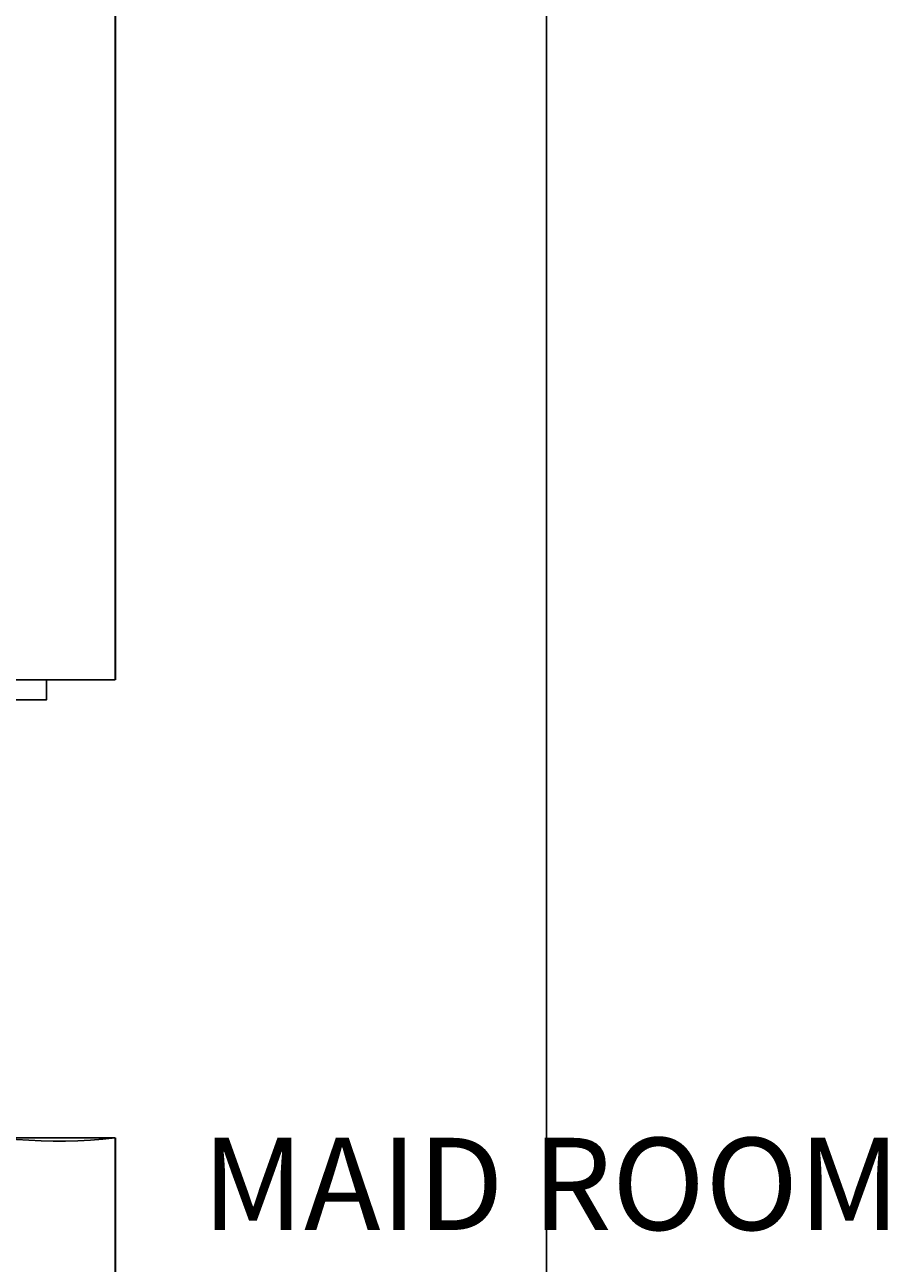
# Model space of a CAD drawing. Units: inches. Extents: x -61 to 1599, y -1316 to 257.
# Tile 85 of 204: x 321 to 367, y -407 to -342. Entities that reach past the tile are written whole.
import ezdxf

# ---------------------------------------------------------------- set-up
doc = ezdxf.new("R2010")
doc.units = ezdxf.units.IN
doc.header["$MEASUREMENT"] = 0
doc.linetypes.add('ACAD_ISO02W100', pattern=[15, 12, -3])
for name, color, linetype, lineweight in [('A-ANNO-DIMS', 2, 'Continuous', 18), ('A-AREA-IDEN', 1, 'Continuous', 18), ('A-WALL-JAMB', 4, 'ACAD_ISO02W100', 25), ('DOORS', 2, 'Continuous', 25), ('WALLS', 4, 'Continuous', 35)]:
    doc.layers.add(name, color=color, linetype=linetype, lineweight=lineweight)
doc.styles.get("Standard").update_dxf_attribs({"font": 'arial.ttf'})
doc.dimstyles.get("Standard").update_dxf_attribs({"dimtxt": 0.18, "dimasz": 0.18, "dimexe": 0.18, "dimexo": 0.0625, "dimgap": 0.09, "dimtad": 0, "dimtih": 1, "dimtoh": 1, "dimdec": 0, "dimzin": 0, "dimdsep": 46, "dimlunit": 3, "dimtxsty": 'Standard', "dimcen": 0.09, "dimadec": 0, "dimazin": 0, "dimtfac": 1, "dimtdec": 0, "dimtofl": 0, "dimtmove": 0, "dimatfit": 3, "dimfxl": 1, "dimtolj": 1, "dimtzin": 0, "dimarcsym": 0})

# ---------------------------------------------------------------- blocks, each defined once
blk = doc.blocks.new('DOOR-SWING-24')
blk.add_line((0, 0), (0, 3.6))
blk.add_lwpolyline([(0, 0), (0, -24), (1.05, -24), (1.05, 0)], close=True)
blk.add_arc((-0.441, 0.618), 24.622, 271.02591, 6.95592)
blk = doc.blocks.new('*D699')
at = {"layer": 'A-ANNO-DIMS', "color": 0, "lineweight": -2, "transparency": 16777216}
for p, q in [((835.64, -167.169), (-61.077, -167.169)), ((-60.897, -167.349), (-60.897, -306.726)), ((-60.897, -446.466), (-60.897, -307.09)), ((841.64, -446.646), (-61.077, -446.646))]:
    blk.add_line(p, q, dxfattribs=at)
at = {"layer": 'A-ANNO-DIMS', "color": 0, "transparency": 16777216}
for points in [[(-60.927, -167.349), (-60.867, -167.349), (-60.897, -167.169)], [(-60.927, -446.466), (-60.867, -446.466), (-60.897, -446.646)]]:
    blk.add_solid(points, dxfattribs=at)
at = {"layer": 'DEFPOINTS', "color": 0, "transparency": 16777216}
for p in [(835.703, -167.169), (-60.897, -446.646), (841.703, -446.646)]:
    blk.add_point(p, dxfattribs=at)
at = {"layer": 'A-ANNO-DIMS', "color": 0, "transparency": 16777216, "insert": (-60.897, -306.908), "char_height": 0.18, "attachment_point": 5}
blk.add_mtext('\\A1;279.5', dxfattribs=at)
blk = doc.blocks.new('*D702')
at = {"layer": 'A-ANNO-DIMS', "color": 0, "lineweight": -2, "transparency": 16777216}
for p, q in [((276.882, -616.882), (276.882, 257.457)), ((277.062, 257.277), (312.209, 257.277)), ((348.14, 257.277), (312.994, 257.277)), ((348.32, -616.882), (348.32, 257.457))]:
    blk.add_line(p, q, dxfattribs=at)
at = {"layer": 'A-ANNO-DIMS', "color": 0, "transparency": 16777216}
for points in [[(277.062, 257.307), (277.062, 257.247), (276.882, 257.277)], [(348.14, 257.307), (348.14, 257.247), (348.32, 257.277)]]:
    blk.add_solid(points, dxfattribs=at)
at = {"layer": 'DEFPOINTS', "color": 0, "transparency": 16777216}
for p in [(348.32, 257.277), (276.882, -616.945), (348.32, -616.945)]:
    blk.add_point(p, dxfattribs=at)
at = {"layer": 'A-ANNO-DIMS', "color": 0, "transparency": 16777216, "insert": (312.601, 257.277), "char_height": 0.18, "attachment_point": 5}
blk.add_mtext('\\A1;71.44', dxfattribs=at)

msp = doc.modelspace()

# ---------------------------------------------------------------- linework, layer by layer
at = {"layer": 'A-WALL-JAMB'}
for p, q in [((325.7028, -376.2211), (319.7028, -376.2211)), ((325.7028, -400.2211), (319.7028, -400.2211))]:
    msp.add_line(p, q, dxfattribs=at)
at = {"layer": 'WALLS'}
for p, q in [((325.7028, -310.3229), (325.7028, -376.2211)), ((325.7028, -400.2211), (325.7028, -441.3229))]:
    msp.add_line(p, q, dxfattribs=at)

# ---------------------------------------------------------------- block references
at = {"layer": 'DOORS', "rotation": 270}
msp.add_blockref('DOOR-SWING-24', (322.1028, -376.2211), dxfattribs=at)

# ---------------------------------------------------------------- texts
at = {"layer": 'A-AREA-IDEN'}
msp.add_text('MAID ROOM', height=4.8321, dxfattribs=at).set_placement((330.2598, -405.0558))

# ---------------------------------------------------------------- dimensions: what is measured, and where the dimension line sits
at = {"layer": 'A-ANNO-DIMS'}
dim = msp.add_linear_dim(base=(348.3201, 257.2771), p1=(276.8825, -616.9446), p2=(348.3201, -616.9446), dimstyle='Standard', override={"dimdec": 2, "dimlfac": 1, "dimrnd": 0, "dimzin": 0, "dimdsep": 46, "dimlunit": 2}, dxfattribs=at)
dim.commit()
dim.dimension.update_dxf_attribs({"geometry": '*D702', "text_midpoint": (312.6013, 257.2771)})
dim = msp.add_linear_dim(base=(-60.8972, -446.6462), p1=(835.7028, -167.169), p2=(841.7028, -446.6462), angle=90, dimstyle='Standard', override={"dimdec": 1, "dimlfac": 1, "dimrnd": 0, "dimzin": 0, "dimdsep": 46, "dimlunit": 2}, dxfattribs=at)
dim.commit()
dim.dimension.update_dxf_attribs({"geometry": '*D699', "text_midpoint": (-60.8972, -306.9076)})

doc.saveas('drawing.dxf')
